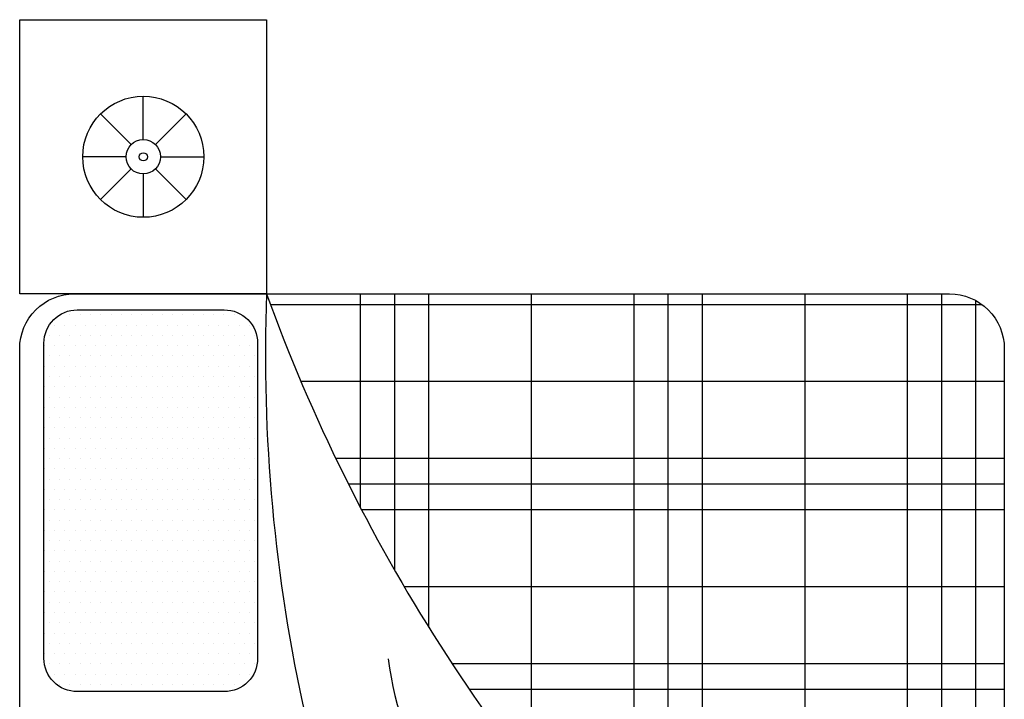
# Model space of a CAD drawing. Units: inches. Extents: x 528 to 2520, y -151 to 1354.
# Tile 33 of 41: x 2171 to 2226, y 770 to 808. Entities that reach past the tile are written whole.
import ezdxf

# ---------------------------------------------------------------- set-up
doc = ezdxf.new("R2010")
doc.units = ezdxf.units.IN
doc.header["$MEASUREMENT"] = 0
doc.layers.add('A-FURN', color=8, linetype='Continuous', lineweight=18)
doc.layers.add('BLOCK', color=6, linetype='Continuous')

# ---------------------------------------------------------------- blocks, each defined once
blk = doc.blocks.new('*X15')
at = {"color": 0}
for p, q in [((276.598, 451.25), (280.51, 451.25)), ((275.455, 450.625), (280.51, 450.625)), ((274.411, 450), (280.51, 450)), ((265.51, 448.125), (267.634, 448.125)), ((271.723, 448.125), (280.51, 448.125)), ((265.51, 446.25), (268.465, 446.25)), ((269.519, 446.25), (280.51, 446.25)), ((265.51, 445.625), (268.531, 445.625)), ((268.866, 445.625), (280.51, 445.625)), ((265.51, 445), (280.51, 445)), ((265.51, 443.125), (280.51, 443.125)), ((265.51, 441.25), (280.51, 441.25)), ((265.51, 440.625), (280.51, 440.625)), ((265.634, 440), (280.386, 440))]:
    blk.add_line(p, q, dxfattribs=at)
blk = doc.blocks.new('*X16')
at = {"color": 0}
for p, q in [((280.312, 439.886), (280.312, 452.896)), ((278.906, 439.482), (278.906, 452.338)), ((277.5, 439.482), (277.5, 451.702)), ((277.031, 439.482), (277.031, 451.471)), ((276.562, 439.482), (276.562, 451.231)), ((275.156, 439.482), (275.156, 450.451)), ((265.781, 439.797), (265.781, 449.511)), ((273.75, 439.482), (273.75, 449.576)), ((266.25, 439.517), (266.25, 449.296)), ((273.281, 439.482), (273.281, 449.261)), ((272.812, 439.482), (272.812, 448.934)), ((267.656, 439.482), (267.656, 448.095)), ((271.406, 439.482), (271.406, 447.876)), ((270, 439.482), (270, 446.689)), ((269.531, 439.482), (269.531, 446.262)), ((269.062, 439.482), (269.062, 445.817))]:
    blk.add_line(p, q, dxfattribs=at)
blk = doc.blocks.new('*X17')
at = {"color": 0}
for p, q in [((273.9375, 457.03125), (273.9375, 457.03125)), ((274.3125, 457.03125), (274.3125, 457.03125)), ((274.6875, 457.03125), (274.6875, 457.03125)), ((275.0625, 457.03125), (275.0625, 457.03125)), ((275.4375, 457.03125), (275.4375, 457.03125)), ((275.8125, 457.03125), (275.8125, 457.03125)), ((276.1875, 457.03125), (276.1875, 457.03125)), ((276.5625, 457.03125), (276.5625, 457.03125)), ((276.9375, 457.03125), (276.9375, 457.03125)), ((277.3125, 457.03125), (277.3125, 457.03125)), ((277.6875, 457.03125), (277.6875, 457.03125)), ((278.0625, 457.03125), (278.0625, 457.03125)), ((278.4375, 457.03125), (278.4375, 457.03125)), ((278.8125, 457.03125), (278.8125, 457.03125)), ((279.1875, 457.03125), (279.1875, 457.03125)), ((279.5625, 457.03125), (279.5625, 457.03125)), ((273.5625, 456.84375), (273.5625, 456.84375)), ((273.75, 456.9375), (273.75, 456.9375)), ((273.9375, 456.84375), (273.9375, 456.84375)), ((274.125, 456.9375), (274.125, 456.9375)), ((274.3125, 456.84375), (274.3125, 456.84375)), ((274.5, 456.9375), (274.5, 456.9375)), ((274.6875, 456.84375), (274.6875, 456.84375)), ((274.875, 456.9375), (274.875, 456.9375)), ((275.0625, 456.84375), (275.0625, 456.84375)), ((275.25, 456.9375), (275.25, 456.9375)), ((275.4375, 456.84375), (275.4375, 456.84375)), ((275.625, 456.9375), (275.625, 456.9375)), ((275.8125, 456.84375), (275.8125, 456.84375)), ((276, 456.9375), (276, 456.9375)), ((276.1875, 456.84375), (276.1875, 456.84375)), ((276.375, 456.9375), (276.375, 456.9375)), ((276.5625, 456.84375), (276.5625, 456.84375)), ((276.75, 456.9375), (276.75, 456.9375)), ((276.9375, 456.84375), (276.9375, 456.84375)), ((277.125, 456.9375), (277.125, 456.9375)), ((277.3125, 456.84375), (277.3125, 456.84375)), ((277.5, 456.9375), (277.5, 456.9375)), ((277.6875, 456.84375), (277.6875, 456.84375)), ((277.875, 456.9375), (277.875, 456.9375)), ((278.0625, 456.84375), (278.0625, 456.84375)), ((278.25, 456.9375), (278.25, 456.9375)), ((278.4375, 456.84375), (278.4375, 456.84375)), ((278.625, 456.9375), (278.625, 456.9375)), ((278.8125, 456.84375), (278.8125, 456.84375)), ((279, 456.9375), (279, 456.9375)), ((279.1875, 456.84375), (279.1875, 456.84375)), ((279.375, 456.9375), (279.375, 456.9375)), ((279.5625, 456.84375), (279.5625, 456.84375)), ((279.75, 456.9375), (279.75, 456.9375)), ((279.9375, 456.84375), (279.9375, 456.84375)), ((273.375, 456.75), (273.375, 456.75)), ((273.75, 456.75), (273.75, 456.75)), ((274.125, 456.75), (274.125, 456.75)), ((274.5, 456.75), (274.5, 456.75)), ((274.875, 456.75), (274.875, 456.75)), ((275.25, 456.75), (275.25, 456.75)), ((275.625, 456.75), (275.625, 456.75)), ((276, 456.75), (276, 456.75)), ((276.375, 456.75), (276.375, 456.75)), ((276.75, 456.75), (276.75, 456.75)), ((277.125, 456.75), (277.125, 456.75)), ((277.5, 456.75), (277.5, 456.75)), ((277.875, 456.75), (277.875, 456.75)), ((278.25, 456.75), (278.25, 456.75)), ((278.625, 456.75), (278.625, 456.75)), ((279, 456.75), (279, 456.75)), ((279.375, 456.75), (279.375, 456.75)), ((279.75, 456.75), (279.75, 456.75)), ((280.125, 456.75), (280.125, 456.75)), ((273.375, 456.5625), (273.375, 456.5625)), ((273.5625, 456.65625), (273.5625, 456.65625)), ((273.75, 456.5625), (273.75, 456.5625)), ((273.9375, 456.65625), (273.9375, 456.65625)), ((274.125, 456.5625), (274.125, 456.5625)), ((274.3125, 456.65625), (274.3125, 456.65625)), ((274.5, 456.5625), (274.5, 456.5625)), ((274.6875, 456.65625), (274.6875, 456.65625)), ((274.875, 456.5625), (274.875, 456.5625)), ((275.0625, 456.65625), (275.0625, 456.65625)), ((275.25, 456.5625), (275.25, 456.5625)), ((275.4375, 456.65625), (275.4375, 456.65625)), ((275.625, 456.5625), (275.625, 456.5625)), ((275.8125, 456.65625), (275.8125, 456.65625)), ((276, 456.5625), (276, 456.5625)), ((276.1875, 456.65625), (276.1875, 456.65625)), ((276.375, 456.5625), (276.375, 456.5625)), ((276.5625, 456.65625), (276.5625, 456.65625)), ((276.75, 456.5625), (276.75, 456.5625)), ((276.9375, 456.65625), (276.9375, 456.65625)), ((277.125, 456.5625), (277.125, 456.5625)), ((277.3125, 456.65625), (277.3125, 456.65625)), ((277.5, 456.5625), (277.5, 456.5625)), ((277.6875, 456.65625), (277.6875, 456.65625)), ((277.875, 456.5625), (277.875, 456.5625)), ((278.0625, 456.65625), (278.0625, 456.65625)), ((278.25, 456.5625), (278.25, 456.5625)), ((278.4375, 456.65625), (278.4375, 456.65625)), ((278.625, 456.5625), (278.625, 456.5625)), ((278.8125, 456.65625), (278.8125, 456.65625)), ((279, 456.5625), (279, 456.5625)), ((279.1875, 456.65625), (279.1875, 456.65625)), ((279.375, 456.5625), (279.375, 456.5625)), ((279.5625, 456.65625), (279.5625, 456.65625)), ((279.75, 456.5625), (279.75, 456.5625)), ((279.9375, 456.65625), (279.9375, 456.65625)), ((280.125, 456.5625), (280.125, 456.5625)), ((273.375, 456.375), (273.375, 456.375)), ((273.5625, 456.46875), (273.5625, 456.46875)), ((273.75, 456.375), (273.75, 456.375)), ((273.9375, 456.46875), (273.9375, 456.46875)), ((274.125, 456.375), (274.125, 456.375)), ((274.3125, 456.46875), (274.3125, 456.46875)), ((274.5, 456.375), (274.5, 456.375)), ((274.6875, 456.46875), (274.6875, 456.46875)), ((274.875, 456.375), (274.875, 456.375)), ((275.0625, 456.46875), (275.0625, 456.46875)), ((275.25, 456.375), (275.25, 456.375)), ((275.4375, 456.46875), (275.4375, 456.46875)), ((275.625, 456.375), (275.625, 456.375)), ((275.8125, 456.46875), (275.8125, 456.46875)), ((276, 456.375), (276, 456.375)), ((276.1875, 456.46875), (276.1875, 456.46875)), ((276.375, 456.375), (276.375, 456.375)), ((276.5625, 456.46875), (276.5625, 456.46875)), ((276.75, 456.375), (276.75, 456.375)), ((276.9375, 456.46875), (276.9375, 456.46875)), ((277.125, 456.375), (277.125, 456.375)), ((277.3125, 456.46875), (277.3125, 456.46875)), ((277.5, 456.375), (277.5, 456.375)), ((277.6875, 456.46875), (277.6875, 456.46875)), ((277.875, 456.375), (277.875, 456.375)), ((278.0625, 456.46875), (278.0625, 456.46875)), ((278.25, 456.375), (278.25, 456.375)), ((278.4375, 456.46875), (278.4375, 456.46875)), ((278.625, 456.375), (278.625, 456.375)), ((278.8125, 456.46875), (278.8125, 456.46875)), ((279, 456.375), (279, 456.375)), ((279.1875, 456.46875), (279.1875, 456.46875)), ((279.375, 456.375), (279.375, 456.375)), ((279.5625, 456.46875), (279.5625, 456.46875)), ((279.75, 456.375), (279.75, 456.375)), ((279.9375, 456.46875), (279.9375, 456.46875)), ((280.125, 456.375), (280.125, 456.375)), ((273.375, 456.1875), (273.375, 456.1875)), ((273.5625, 456.28125), (273.5625, 456.28125)), ((273.75, 456.1875), (273.75, 456.1875)), ((273.9375, 456.28125), (273.9375, 456.28125)), ((274.125, 456.1875), (274.125, 456.1875)), ((274.3125, 456.28125), (274.3125, 456.28125)), ((274.5, 456.1875), (274.5, 456.1875)), ((274.6875, 456.28125), (274.6875, 456.28125)), ((274.875, 456.1875), (274.875, 456.1875)), ((275.0625, 456.28125), (275.0625, 456.28125)), ((275.25, 456.1875), (275.25, 456.1875)), ((275.4375, 456.28125), (275.4375, 456.28125)), ((275.625, 456.1875), (275.625, 456.1875)), ((275.8125, 456.28125), (275.8125, 456.28125)), ((276, 456.1875), (276, 456.1875)), ((276.1875, 456.28125), (276.1875, 456.28125)), ((276.375, 456.1875), (276.375, 456.1875)), ((276.5625, 456.28125), (276.5625, 456.28125)), ((276.75, 456.1875), (276.75, 456.1875)), ((276.9375, 456.28125), (276.9375, 456.28125)), ((277.125, 456.1875), (277.125, 456.1875)), ((277.3125, 456.28125), (277.3125, 456.28125)), ((277.5, 456.1875), (277.5, 456.1875)), ((277.6875, 456.28125), (277.6875, 456.28125)), ((277.875, 456.1875), (277.875, 456.1875)), ((278.0625, 456.28125), (278.0625, 456.28125)), ((278.25, 456.1875), (278.25, 456.1875)), ((278.4375, 456.28125), (278.4375, 456.28125)), ((278.625, 456.1875), (278.625, 456.1875)), ((278.8125, 456.28125), (278.8125, 456.28125)), ((279, 456.1875), (279, 456.1875)), ((279.1875, 456.28125), (279.1875, 456.28125)), ((279.375, 456.1875), (279.375, 456.1875)), ((279.5625, 456.28125), (279.5625, 456.28125)), ((279.75, 456.1875), (279.75, 456.1875)), ((279.9375, 456.28125), (279.9375, 456.28125)), ((280.125, 456.1875), (280.125, 456.1875)), ((273.375, 456), (273.375, 456)), ((273.5625, 456.09375), (273.5625, 456.09375)), ((273.75, 456), (273.75, 456)), ((273.9375, 456.09375), (273.9375, 456.09375)), ((274.125, 456), (274.125, 456)), ((274.3125, 456.09375), (274.3125, 456.09375)), ((274.5, 456), (274.5, 456)), ((274.6875, 456.09375), (274.6875, 456.09375)), ((274.875, 456), (274.875, 456)), ((275.0625, 456.09375), (275.0625, 456.09375)), ((275.25, 456), (275.25, 456)), ((275.4375, 456.09375), (275.4375, 456.09375)), ((275.625, 456), (275.625, 456)), ((275.8125, 456.09375), (275.8125, 456.09375)), ((276, 456), (276, 456)), ((276.1875, 456.09375), (276.1875, 456.09375)), ((276.375, 456), (276.375, 456)), ((276.5625, 456.09375), (276.5625, 456.09375)), ((276.75, 456), (276.75, 456)), ((276.9375, 456.09375), (276.9375, 456.09375)), ((277.125, 456), (277.125, 456)), ((277.3125, 456.09375), (277.3125, 456.09375)), ((277.5, 456), (277.5, 456)), ((277.6875, 456.09375), (277.6875, 456.09375)), ((277.875, 456), (277.875, 456)), ((278.0625, 456.09375), (278.0625, 456.09375)), ((278.25, 456), (278.25, 456)), ((278.4375, 456.09375), (278.4375, 456.09375)), ((278.625, 456), (278.625, 456)), ((278.8125, 456.09375), (278.8125, 456.09375)), ((279, 456), (279, 456)), ((279.1875, 456.09375), (279.1875, 456.09375)), ((279.375, 456), (279.375, 456)), ((279.5625, 456.09375), (279.5625, 456.09375)), ((279.75, 456), (279.75, 456)), ((279.9375, 456.09375), (279.9375, 456.09375)), ((280.125, 456), (280.125, 456)), ((273.375, 455.8125), (273.375, 455.8125)), ((273.5625, 455.90625), (273.5625, 455.90625)), ((273.75, 455.8125), (273.75, 455.8125)), ((273.9375, 455.90625), (273.9375, 455.90625)), ((274.125, 455.8125), (274.125, 455.8125)), ((274.3125, 455.90625), (274.3125, 455.90625)), ((274.5, 455.8125), (274.5, 455.8125)), ((274.6875, 455.90625), (274.6875, 455.90625)), ((274.875, 455.8125), (274.875, 455.8125)), ((275.0625, 455.90625), (275.0625, 455.90625)), ((275.25, 455.8125), (275.25, 455.8125)), ((275.4375, 455.90625), (275.4375, 455.90625)), ((275.625, 455.8125), (275.625, 455.8125)), ((275.8125, 455.90625), (275.8125, 455.90625)), ((276, 455.8125), (276, 455.8125)), ((276.1875, 455.90625), (276.1875, 455.90625)), ((276.375, 455.8125), (276.375, 455.8125)), ((276.5625, 455.90625), (276.5625, 455.90625)), ((276.75, 455.8125), (276.75, 455.8125)), ((276.9375, 455.90625), (276.9375, 455.90625)), ((277.125, 455.8125), (277.125, 455.8125)), ((277.3125, 455.90625), (277.3125, 455.90625)), ((277.5, 455.8125), (277.5, 455.8125)), ((277.6875, 455.90625), (277.6875, 455.90625)), ((277.875, 455.8125), (277.875, 455.8125)), ((278.0625, 455.90625), (278.0625, 455.90625)), ((278.25, 455.8125), (278.25, 455.8125)), ((278.4375, 455.90625), (278.4375, 455.90625)), ((278.625, 455.8125), (278.625, 455.8125)), ((278.8125, 455.90625), (278.8125, 455.90625)), ((279, 455.8125), (279, 455.8125)), ((279.1875, 455.90625), (279.1875, 455.90625)), ((279.375, 455.8125), (279.375, 455.8125)), ((279.5625, 455.90625), (279.5625, 455.90625)), ((279.75, 455.8125), (279.75, 455.8125)), ((279.9375, 455.90625), (279.9375, 455.90625)), ((280.125, 455.8125), (280.125, 455.8125)), ((273.375, 455.625), (273.375, 455.625)), ((273.5625, 455.71875), (273.5625, 455.71875)), ((273.75, 455.625), (273.75, 455.625)), ((273.9375, 455.71875), (273.9375, 455.71875)), ((274.125, 455.625), (274.125, 455.625)), ((274.3125, 455.71875), (274.3125, 455.71875)), ((274.5, 455.625), (274.5, 455.625)), ((274.6875, 455.71875), (274.6875, 455.71875)), ((274.875, 455.625), (274.875, 455.625)), ((275.0625, 455.71875), (275.0625, 455.71875)), ((275.25, 455.625), (275.25, 455.625)), ((275.4375, 455.71875), (275.4375, 455.71875)), ((275.625, 455.625), (275.625, 455.625)), ((275.8125, 455.71875), (275.8125, 455.71875)), ((276, 455.625), (276, 455.625)), ((276.1875, 455.71875), (276.1875, 455.71875)), ((276.375, 455.625), (276.375, 455.625)), ((276.5625, 455.71875), (276.5625, 455.71875)), ((276.75, 455.625), (276.75, 455.625)), ((276.9375, 455.71875), (276.9375, 455.71875)), ((277.125, 455.625), (277.125, 455.625)), ((277.3125, 455.71875), (277.3125, 455.71875)), ((277.5, 455.625), (277.5, 455.625)), ((277.6875, 455.71875), (277.6875, 455.71875)), ((277.875, 455.625), (277.875, 455.625)), ((278.0625, 455.71875), (278.0625, 455.71875)), ((278.25, 455.625), (278.25, 455.625)), ((278.4375, 455.71875), (278.4375, 455.71875)), ((278.625, 455.625), (278.625, 455.625)), ((278.8125, 455.71875), (278.8125, 455.71875)), ((279, 455.625), (279, 455.625)), ((279.1875, 455.71875), (279.1875, 455.71875)), ((279.375, 455.625), (279.375, 455.625)), ((279.5625, 455.71875), (279.5625, 455.71875)), ((279.75, 455.625), (279.75, 455.625)), ((279.9375, 455.71875), (279.9375, 455.71875)), ((280.125, 455.625), (280.125, 455.625)), ((273.375, 455.4375), (273.375, 455.4375)), ((273.5625, 455.53125), (273.5625, 455.53125)), ((273.75, 455.4375), (273.75, 455.4375)), ((273.9375, 455.53125), (273.9375, 455.53125)), ((274.125, 455.4375), (274.125, 455.4375)), ((274.3125, 455.53125), (274.3125, 455.53125)), ((274.5, 455.4375), (274.5, 455.4375)), ((274.6875, 455.53125), (274.6875, 455.53125)), ((274.875, 455.4375), (274.875, 455.4375)), ((275.0625, 455.53125), (275.0625, 455.53125)), ((275.25, 455.4375), (275.25, 455.4375)), ((275.4375, 455.53125), (275.4375, 455.53125)), ((275.625, 455.4375), (275.625, 455.4375)), ((275.8125, 455.53125), (275.8125, 455.53125)), ((276, 455.4375), (276, 455.4375)), ((276.1875, 455.53125), (276.1875, 455.53125)), ((276.375, 455.4375), (276.375, 455.4375)), ((276.5625, 455.53125), (276.5625, 455.53125)), ((276.75, 455.4375), (276.75, 455.4375)), ((276.9375, 455.53125), (276.9375, 455.53125)), ((277.125, 455.4375), (277.125, 455.4375)), ((277.3125, 455.53125), (277.3125, 455.53125)), ((277.5, 455.4375), (277.5, 455.4375)), ((277.6875, 455.53125), (277.6875, 455.53125)), ((277.875, 455.4375), (277.875, 455.4375)), ((278.0625, 455.53125), (278.0625, 455.53125)), ((278.25, 455.4375), (278.25, 455.4375)), ((278.4375, 455.53125), (278.4375, 455.53125)), ((278.625, 455.4375), (278.625, 455.4375)), ((278.8125, 455.53125), (278.8125, 455.53125)), ((279, 455.4375), (279, 455.4375)), ((279.1875, 455.53125), (279.1875, 455.53125)), ((279.375, 455.4375), (279.375, 455.4375)), ((279.5625, 455.53125), (279.5625, 455.53125)), ((279.75, 455.4375), (279.75, 455.4375)), ((279.9375, 455.53125), (279.9375, 455.53125)), ((280.125, 455.4375), (280.125, 455.4375)), ((273.375, 455.25), (273.375, 455.25)), ((273.5625, 455.34375), (273.5625, 455.34375)), ((273.75, 455.25), (273.75, 455.25)), ((273.9375, 455.34375), (273.9375, 455.34375)), ((274.125, 455.25), (274.125, 455.25)), ((274.3125, 455.34375), (274.3125, 455.34375)), ((274.5, 455.25), (274.5, 455.25)), ((274.6875, 455.34375), (274.6875, 455.34375)), ((274.875, 455.25), (274.875, 455.25)), ((275.0625, 455.34375), (275.0625, 455.34375)), ((275.25, 455.25), (275.25, 455.25)), ((275.4375, 455.34375), (275.4375, 455.34375)), ((275.625, 455.25), (275.625, 455.25)), ((275.8125, 455.34375), (275.8125, 455.34375)), ((276, 455.25), (276, 455.25)), ((276.1875, 455.34375), (276.1875, 455.34375)), ((276.375, 455.25), (276.375, 455.25)), ((276.5625, 455.34375), (276.5625, 455.34375)), ((276.75, 455.25), (276.75, 455.25)), ((276.9375, 455.34375), (276.9375, 455.34375)), ((277.125, 455.25), (277.125, 455.25)), ((277.3125, 455.34375), (277.3125, 455.34375)), ((277.5, 455.25), (277.5, 455.25)), ((277.6875, 455.34375), (277.6875, 455.34375)), ((277.875, 455.25), (277.875, 455.25)), ((278.0625, 455.34375), (278.0625, 455.34375)), ((278.25, 455.25), (278.25, 455.25)), ((278.4375, 455.34375), (278.4375, 455.34375)), ((278.625, 455.25), (278.625, 455.25)), ((278.8125, 455.34375), (278.8125, 455.34375)), ((279, 455.25), (279, 455.25)), ((279.1875, 455.34375), (279.1875, 455.34375)), ((279.375, 455.25), (279.375, 455.25)), ((279.5625, 455.34375), (279.5625, 455.34375)), ((279.75, 455.25), (279.75, 455.25)), ((279.9375, 455.34375), (279.9375, 455.34375)), ((280.125, 455.25), (280.125, 455.25)), ((273.375, 455.0625), (273.375, 455.0625)), ((273.5625, 455.15625), (273.5625, 455.15625)), ((273.75, 455.0625), (273.75, 455.0625)), ((273.9375, 455.15625), (273.9375, 455.15625)), ((274.125, 455.0625), (274.125, 455.0625)), ((274.3125, 455.15625), (274.3125, 455.15625)), ((274.5, 455.0625), (274.5, 455.0625)), ((274.6875, 455.15625), (274.6875, 455.15625)), ((274.875, 455.0625), (274.875, 455.0625)), ((275.0625, 455.15625), (275.0625, 455.15625)), ((275.25, 455.0625), (275.25, 455.0625)), ((275.4375, 455.15625), (275.4375, 455.15625)), ((275.625, 455.0625), (275.625, 455.0625)), ((275.8125, 455.15625), (275.8125, 455.15625)), ((276, 455.0625), (276, 455.0625)), ((276.1875, 455.15625), (276.1875, 455.15625)), ((276.375, 455.0625), (276.375, 455.0625)), ((276.5625, 455.15625), (276.5625, 455.15625)), ((276.75, 455.0625), (276.75, 455.0625)), ((276.9375, 455.15625), (276.9375, 455.15625)), ((277.125, 455.0625), (277.125, 455.0625)), ((277.3125, 455.15625), (277.3125, 455.15625)), ((277.5, 455.0625), (277.5, 455.0625)), ((277.6875, 455.15625), (277.6875, 455.15625)), ((277.875, 455.0625), (277.875, 455.0625)), ((278.0625, 455.15625), (278.0625, 455.15625)), ((278.25, 455.0625), (278.25, 455.0625)), ((278.4375, 455.15625), (278.4375, 455.15625)), ((278.625, 455.0625), (278.625, 455.0625)), ((278.8125, 455.15625), (278.8125, 455.15625)), ((279, 455.0625), (279, 455.0625)), ((279.1875, 455.15625), (279.1875, 455.15625)), ((279.375, 455.0625), (279.375, 455.0625)), ((279.5625, 455.15625), (279.5625, 455.15625)), ((279.75, 455.0625), (279.75, 455.0625)), ((279.9375, 455.15625), (279.9375, 455.15625)), ((280.125, 455.0625), (280.125, 455.0625)), ((273.375, 454.875), (273.375, 454.875)), ((273.5625, 454.96875), (273.5625, 454.96875)), ((273.75, 454.875), (273.75, 454.875)), ((273.9375, 454.96875), (273.9375, 454.96875)), ((274.125, 454.875), (274.125, 454.875)), ((274.3125, 454.96875), (274.3125, 454.96875)), ((274.5, 454.875), (274.5, 454.875)), ((274.6875, 454.96875), (274.6875, 454.96875)), ((274.875, 454.875), (274.875, 454.875)), ((275.0625, 454.96875), (275.0625, 454.96875)), ((275.25, 454.875), (275.25, 454.875)), ((275.4375, 454.96875), (275.4375, 454.96875)), ((275.625, 454.875), (275.625, 454.875)), ((275.8125, 454.96875), (275.8125, 454.96875)), ((276, 454.875), (276, 454.875)), ((276.1875, 454.96875), (276.1875, 454.96875)), ((276.375, 454.875), (276.375, 454.875)), ((276.5625, 454.96875), (276.5625, 454.96875)), ((276.75, 454.875), (276.75, 454.875)), ((276.9375, 454.96875), (276.9375, 454.96875)), ((277.125, 454.875), (277.125, 454.875)), ((277.3125, 454.96875), (277.3125, 454.96875)), ((277.5, 454.875), (277.5, 454.875)), ((277.6875, 454.96875), (277.6875, 454.96875)), ((277.875, 454.875), (277.875, 454.875)), ((278.0625, 454.96875), (278.0625, 454.96875)), ((278.25, 454.875), (278.25, 454.875)), ((278.4375, 454.96875), (278.4375, 454.96875)), ((278.625, 454.875), (278.625, 454.875)), ((278.8125, 454.96875), (278.8125, 454.96875)), ((279, 454.875), (279, 454.875)), ((279.1875, 454.96875), (279.1875, 454.96875)), ((279.375, 454.875), (279.375, 454.875)), ((279.5625, 454.96875), (279.5625, 454.96875)), ((279.75, 454.875), (279.75, 454.875)), ((279.9375, 454.96875), (279.9375, 454.96875)), ((280.125, 454.875), (280.125, 454.875)), ((273.375, 454.6875), (273.375, 454.6875)), ((273.5625, 454.78125), (273.5625, 454.78125)), ((273.75, 454.6875), (273.75, 454.6875)), ((273.9375, 454.78125), (273.9375, 454.78125)), ((274.125, 454.6875), (274.125, 454.6875)), ((274.3125, 454.78125), (274.3125, 454.78125)), ((274.5, 454.6875), (274.5, 454.6875)), ((274.6875, 454.78125), (274.6875, 454.78125)), ((274.875, 454.6875), (274.875, 454.6875)), ((275.0625, 454.78125), (275.0625, 454.78125)), ((275.25, 454.6875), (275.25, 454.6875)), ((275.4375, 454.78125), (275.4375, 454.78125)), ((275.625, 454.6875), (275.625, 454.6875)), ((275.8125, 454.78125), (275.8125, 454.78125)), ((276, 454.6875), (276, 454.6875)), ((276.1875, 454.78125), (276.1875, 454.78125)), ((276.375, 454.6875), (276.375, 454.6875)), ((276.5625, 454.78125), (276.5625, 454.78125)), ((276.75, 454.6875), (276.75, 454.6875)), ((276.9375, 454.78125), (276.9375, 454.78125)), ((277.125, 454.6875), (277.125, 454.6875)), ((277.3125, 454.78125), (277.3125, 454.78125)), ((277.5, 454.6875), (277.5, 454.6875)), ((277.6875, 454.78125), (277.6875, 454.78125)), ((277.875, 454.6875), (277.875, 454.6875)), ((278.0625, 454.78125), (278.0625, 454.78125)), ((278.25, 454.6875), (278.25, 454.6875)), ((278.4375, 454.78125), (278.4375, 454.78125)), ((278.625, 454.6875), (278.625, 454.6875)), ((278.8125, 454.78125), (278.8125, 454.78125)), ((279, 454.6875), (279, 454.6875)), ((279.1875, 454.78125), (279.1875, 454.78125)), ((279.375, 454.6875), (279.375, 454.6875)), ((279.5625, 454.78125), (279.5625, 454.78125)), ((279.75, 454.6875), (279.75, 454.6875)), ((279.9375, 454.78125), (279.9375, 454.78125)), ((280.125, 454.6875), (280.125, 454.6875)), ((273.5625, 454.59375), (273.5625, 454.59375)), ((273.9375, 454.59375), (273.9375, 454.59375)), ((274.3125, 454.59375), (274.3125, 454.59375)), ((274.6875, 454.59375), (274.6875, 454.59375)), ((275.0625, 454.59375), (275.0625, 454.59375)), ((275.4375, 454.59375), (275.4375, 454.59375)), ((275.8125, 454.59375), (275.8125, 454.59375)), ((276.1875, 454.59375), (276.1875, 454.59375)), ((276.5625, 454.59375), (276.5625, 454.59375)), ((276.9375, 454.59375), (276.9375, 454.59375)), ((277.3125, 454.59375), (277.3125, 454.59375)), ((277.6875, 454.59375), (277.6875, 454.59375)), ((278.0625, 454.59375), (278.0625, 454.59375)), ((278.4375, 454.59375), (278.4375, 454.59375)), ((278.8125, 454.59375), (278.8125, 454.59375)), ((279.1875, 454.59375), (279.1875, 454.59375)), ((279.5625, 454.59375), (279.5625, 454.59375)), ((279.9375, 454.59375), (279.9375, 454.59375)), ((273.375, 454.5), (273.375, 454.5)), ((273.5625, 454.40625), (273.5625, 454.40625)), ((273.75, 454.5), (273.75, 454.5)), ((273.9375, 454.40625), (273.9375, 454.40625)), ((274.125, 454.5), (274.125, 454.5)), ((274.3125, 454.40625), (274.3125, 454.40625)), ((274.5, 454.5), (274.5, 454.5)), ((274.6875, 454.40625), (274.6875, 454.40625)), ((274.875, 454.5), (274.875, 454.5)), ((275.0625, 454.40625), (275.0625, 454.40625)), ((275.25, 454.5), (275.25, 454.5)), ((275.4375, 454.40625), (275.4375, 454.40625)), ((275.625, 454.5), (275.625, 454.5)), ((275.8125, 454.40625), (275.8125, 454.40625)), ((276, 454.5), (276, 454.5)), ((276.1875, 454.40625), (276.1875, 454.40625)), ((276.375, 454.5), (276.375, 454.5)), ((276.5625, 454.40625), (276.5625, 454.40625)), ((276.75, 454.5), (276.75, 454.5)), ((276.9375, 454.40625), (276.9375, 454.40625)), ((277.125, 454.5), (277.125, 454.5)), ((277.3125, 454.40625), (277.3125, 454.40625)), ((277.5, 454.5), (277.5, 454.5)), ((277.6875, 454.40625), (277.6875, 454.40625)), ((277.875, 454.5), (277.875, 454.5)), ((278.0625, 454.40625), (278.0625, 454.40625)), ((278.25, 454.5), (278.25, 454.5)), ((278.4375, 454.40625), (278.4375, 454.40625)), ((278.625, 454.5), (278.625, 454.5)), ((278.8125, 454.40625), (278.8125, 454.40625)), ((279, 454.5), (279, 454.5)), ((279.1875, 454.40625), (279.1875, 454.40625)), ((279.375, 454.5), (279.375, 454.5)), ((279.5625, 454.40625), (279.5625, 454.40625)), ((279.75, 454.5), (279.75, 454.5)), ((279.9375, 454.40625), (279.9375, 454.40625)), ((280.125, 454.5), (280.125, 454.5)), ((273.375, 454.3125), (273.375, 454.3125)), ((273.5625, 454.21875), (273.5625, 454.21875)), ((273.75, 454.3125), (273.75, 454.3125)), ((273.9375, 454.21875), (273.9375, 454.21875)), ((274.125, 454.3125), (274.125, 454.3125)), ((274.3125, 454.21875), (274.3125, 454.21875)), ((274.5, 454.3125), (274.5, 454.3125)), ((274.6875, 454.21875), (274.6875, 454.21875)), ((274.875, 454.3125), (274.875, 454.3125)), ((275.0625, 454.21875), (275.0625, 454.21875)), ((275.25, 454.3125), (275.25, 454.3125)), ((275.4375, 454.21875), (275.4375, 454.21875)), ((275.625, 454.3125), (275.625, 454.3125)), ((275.8125, 454.21875), (275.8125, 454.21875)), ((276, 454.3125), (276, 454.3125)), ((276.1875, 454.21875), (276.1875, 454.21875)), ((276.375, 454.3125), (276.375, 454.3125)), ((276.5625, 454.21875), (276.5625, 454.21875)), ((276.75, 454.3125), (276.75, 454.3125)), ((276.9375, 454.21875), (276.9375, 454.21875)), ((277.125, 454.3125), (277.125, 454.3125)), ((277.3125, 454.21875), (277.3125, 454.21875)), ((277.5, 454.3125), (277.5, 454.3125)), ((277.6875, 454.21875), (277.6875, 454.21875)), ((277.875, 454.3125), (277.875, 454.3125)), ((278.0625, 454.21875), (278.0625, 454.21875)), ((278.25, 454.3125), (278.25, 454.3125)), ((278.4375, 454.21875), (278.4375, 454.21875)), ((278.625, 454.3125), (278.625, 454.3125)), ((278.8125, 454.21875), (278.8125, 454.21875)), ((279, 454.3125), (279, 454.3125)), ((279.1875, 454.21875), (279.1875, 454.21875)), ((279.375, 454.3125), (279.375, 454.3125)), ((279.5625, 454.21875), (279.5625, 454.21875)), ((279.75, 454.3125), (279.75, 454.3125)), ((279.9375, 454.21875), (279.9375, 454.21875)), ((280.125, 454.3125), (280.125, 454.3125)), ((273.375, 454.125), (273.375, 454.125)), ((273.5625, 454.03125), (273.5625, 454.03125)), ((273.75, 454.125), (273.75, 454.125)), ((273.9375, 454.03125), (273.9375, 454.03125)), ((274.125, 454.125), (274.125, 454.125)), ((274.3125, 454.03125), (274.3125, 454.03125)), ((274.5, 454.125), (274.5, 454.125)), ((274.6875, 454.03125), (274.6875, 454.03125)), ((274.875, 454.125), (274.875, 454.125)), ((275.0625, 454.03125), (275.0625, 454.03125)), ((275.25, 454.125), (275.25, 454.125)), ((275.4375, 454.03125), (275.4375, 454.03125)), ((275.625, 454.125), (275.625, 454.125)), ((275.8125, 454.03125), (275.8125, 454.03125)), ((276, 454.125), (276, 454.125)), ((276.1875, 454.03125), (276.1875, 454.03125)), ((276.375, 454.125), (276.375, 454.125)), ((276.5625, 454.03125), (276.5625, 454.03125)), ((276.75, 454.125), (276.75, 454.125)), ((276.9375, 454.03125), (276.9375, 454.03125)), ((277.125, 454.125), (277.125, 454.125)), ((277.3125, 454.03125), (277.3125, 454.03125)), ((277.5, 454.125), (277.5, 454.125)), ((277.6875, 454.03125), (277.6875, 454.03125)), ((277.875, 454.125), (277.875, 454.125)), ((278.0625, 454.03125), (278.0625, 454.03125)), ((278.25, 454.125), (278.25, 454.125)), ((278.4375, 454.03125), (278.4375, 454.03125)), ((278.625, 454.125), (278.625, 454.125)), ((278.8125, 454.03125), (278.8125, 454.03125)), ((279, 454.125), (279, 454.125)), ((279.1875, 454.03125), (279.1875, 454.03125)), ((279.375, 454.125), (279.375, 454.125)), ((279.5625, 454.03125), (279.5625, 454.03125)), ((279.75, 454.125), (279.75, 454.125)), ((279.9375, 454.03125), (279.9375, 454.03125)), ((280.125, 454.125), (280.125, 454.125)), ((273.375, 453.9375), (273.375, 453.9375)), ((273.5625, 453.84375), (273.5625, 453.84375)), ((273.75, 453.9375), (273.75, 453.9375)), ((273.9375, 453.84375), (273.9375, 453.84375)), ((274.125, 453.9375), (274.125, 453.9375)), ((274.3125, 453.84375), (274.3125, 453.84375)), ((274.5, 453.9375), (274.5, 453.9375)), ((274.6875, 453.84375), (274.6875, 453.84375)), ((274.875, 453.9375), (274.875, 453.9375)), ((275.0625, 453.84375), (275.0625, 453.84375)), ((275.25, 453.9375), (275.25, 453.9375)), ((275.4375, 453.84375), (275.4375, 453.84375)), ((275.625, 453.9375), (275.625, 453.9375)), ((275.8125, 453.84375), (275.8125, 453.84375)), ((276, 453.9375), (276, 453.9375)), ((276.1875, 453.84375), (276.1875, 453.84375)), ((276.375, 453.9375), (276.375, 453.9375)), ((276.5625, 453.84375), (276.5625, 453.84375)), ((276.75, 453.9375), (276.75, 453.9375)), ((276.9375, 453.84375), (276.9375, 453.84375)), ((277.125, 453.9375), (277.125, 453.9375)), ((277.3125, 453.84375), (277.3125, 453.84375)), ((277.5, 453.9375), (277.5, 453.9375)), ((277.6875, 453.84375), (277.6875, 453.84375)), ((277.875, 453.9375), (277.875, 453.9375)), ((278.0625, 453.84375), (278.0625, 453.84375)), ((278.25, 453.9375), (278.25, 453.9375)), ((278.4375, 453.84375), (278.4375, 453.84375)), ((278.625, 453.9375), (278.625, 453.9375)), ((278.8125, 453.84375), (278.8125, 453.84375)), ((279, 453.9375), (279, 453.9375)), ((279.1875, 453.84375), (279.1875, 453.84375)), ((279.375, 453.9375), (279.375, 453.9375)), ((279.5625, 453.84375), (279.5625, 453.84375)), ((279.75, 453.9375), (279.75, 453.9375)), ((279.9375, 453.84375), (279.9375, 453.84375)), ((280.125, 453.9375), (280.125, 453.9375)), ((273.375, 453.75), (273.375, 453.75)), ((273.5625, 453.65625), (273.5625, 453.65625)), ((273.75, 453.75), (273.75, 453.75)), ((273.9375, 453.65625), (273.9375, 453.65625)), ((274.125, 453.75), (274.125, 453.75)), ((274.3125, 453.65625), (274.3125, 453.65625)), ((274.5, 453.75), (274.5, 453.75)), ((274.6875, 453.65625), (274.6875, 453.65625)), ((274.875, 453.75), (274.875, 453.75)), ((275.0625, 453.65625), (275.0625, 453.65625)), ((275.25, 453.75), (275.25, 453.75)), ((275.4375, 453.65625), (275.4375, 453.65625)), ((275.625, 453.75), (275.625, 453.75)), ((275.8125, 453.65625), (275.8125, 453.65625)), ((276, 453.75), (276, 453.75)), ((276.1875, 453.65625), (276.1875, 453.65625)), ((276.375, 453.75), (276.375, 453.75)), ((276.5625, 453.65625), (276.5625, 453.65625)), ((276.75, 453.75), (276.75, 453.75)), ((276.9375, 453.65625), (276.9375, 453.65625)), ((277.125, 453.75), (277.125, 453.75)), ((277.3125, 453.65625), (277.3125, 453.65625)), ((277.5, 453.75), (277.5, 453.75)), ((277.6875, 453.65625), (277.6875, 453.65625)), ((277.875, 453.75), (277.875, 453.75)), ((278.0625, 453.65625), (278.0625, 453.65625)), ((278.25, 453.75), (278.25, 453.75)), ((278.4375, 453.65625), (278.4375, 453.65625)), ((278.625, 453.75), (278.625, 453.75)), ((278.8125, 453.65625), (278.8125, 453.65625)), ((279, 453.75), (279, 453.75)), ((279.1875, 453.65625), (279.1875, 453.65625)), ((279.375, 453.75), (279.375, 453.75)), ((279.5625, 453.65625), (279.5625, 453.65625)), ((279.75, 453.75), (279.75, 453.75)), ((279.9375, 453.65625), (279.9375, 453.65625)), ((280.125, 453.75), (280.125, 453.75)), ((273.375, 453.5625), (273.375, 453.5625)), ((273.5625, 453.46875), (273.5625, 453.46875)), ((273.75, 453.5625), (273.75, 453.5625)), ((273.9375, 453.46875), (273.9375, 453.46875)), ((274.125, 453.5625), (274.125, 453.5625)), ((274.3125, 453.46875), (274.3125, 453.46875)), ((274.5, 453.5625), (274.5, 453.5625)), ((274.6875, 453.46875), (274.6875, 453.46875)), ((274.875, 453.5625), (274.875, 453.5625)), ((275.0625, 453.46875), (275.0625, 453.46875)), ((275.25, 453.5625), (275.25, 453.5625)), ((275.4375, 453.46875), (275.4375, 453.46875)), ((275.625, 453.5625), (275.625, 453.5625)), ((275.8125, 453.46875), (275.8125, 453.46875)), ((276, 453.5625), (276, 453.5625)), ((276.1875, 453.46875), (276.1875, 453.46875)), ((276.375, 453.5625), (276.375, 453.5625)), ((276.5625, 453.46875), (276.5625, 453.46875)), ((276.75, 453.5625), (276.75, 453.5625)), ((276.9375, 453.46875), (276.9375, 453.46875)), ((277.125, 453.5625), (277.125, 453.5625)), ((277.3125, 453.46875), (277.3125, 453.46875)), ((277.5, 453.5625), (277.5, 453.5625)), ((277.6875, 453.46875), (277.6875, 453.46875)), ((277.875, 453.5625), (277.875, 453.5625)), ((278.0625, 453.46875), (278.0625, 453.46875)), ((278.25, 453.5625), (278.25, 453.5625)), ((278.4375, 453.46875), (278.4375, 453.46875)), ((278.625, 453.5625), (278.625, 453.5625)), ((278.8125, 453.46875), (278.8125, 453.46875)), ((279, 453.5625), (279, 453.5625)), ((279.1875, 453.46875), (279.1875, 453.46875)), ((279.375, 453.5625), (279.375, 453.5625)), ((279.5625, 453.46875), (279.5625, 453.46875)), ((279.75, 453.5625), (279.75, 453.5625)), ((279.9375, 453.46875), (279.9375, 453.46875)), ((280.125, 453.5625), (280.125, 453.5625)), ((273.375, 453.375), (273.375, 453.375)), ((273.5625, 453.28125), (273.5625, 453.28125)), ((273.75, 453.375), (273.75, 453.375)), ((273.9375, 453.28125), (273.9375, 453.28125)), ((274.125, 453.375), (274.125, 453.375)), ((274.3125, 453.28125), (274.3125, 453.28125)), ((274.5, 453.375), (274.5, 453.375)), ((274.6875, 453.28125), (274.6875, 453.28125)), ((274.875, 453.375), (274.875, 453.375)), ((275.0625, 453.28125), (275.0625, 453.28125)), ((275.25, 453.375), (275.25, 453.375)), ((275.4375, 453.28125), (275.4375, 453.28125)), ((275.625, 453.375), (275.625, 453.375)), ((275.8125, 453.28125), (275.8125, 453.28125)), ((276, 453.375), (276, 453.375)), ((276.1875, 453.28125), (276.1875, 453.28125)), ((276.375, 453.375), (276.375, 453.375)), ((276.5625, 453.28125), (276.5625, 453.28125)), ((276.75, 453.375), (276.75, 453.375)), ((276.9375, 453.28125), (276.9375, 453.28125)), ((277.125, 453.375), (277.125, 453.375)), ((277.3125, 453.28125), (277.3125, 453.28125)), ((277.5, 453.375), (277.5, 453.375)), ((277.6875, 453.28125), (277.6875, 453.28125)), ((277.875, 453.375), (277.875, 453.375)), ((278.0625, 453.28125), (278.0625, 453.28125)), ((278.25, 453.375), (278.25, 453.375)), ((278.4375, 453.28125), (278.4375, 453.28125)), ((278.625, 453.375), (278.625, 453.375)), ((278.8125, 453.28125), (278.8125, 453.28125)), ((279, 453.375), (279, 453.375)), ((279.1875, 453.28125), (279.1875, 453.28125)), ((279.375, 453.375), (279.375, 453.375)), ((279.5625, 453.28125), (279.5625, 453.28125)), ((279.75, 453.375), (279.75, 453.375)), ((279.9375, 453.28125), (279.9375, 453.28125)), ((273.75, 453.1875), (273.75, 453.1875)), ((274.125, 453.1875), (274.125, 453.1875)), ((274.5, 453.1875), (274.5, 453.1875)), ((274.875, 453.1875), (274.875, 453.1875)), ((275.25, 453.1875), (275.25, 453.1875)), ((275.625, 453.1875), (275.625, 453.1875)), ((276, 453.1875), (276, 453.1875)), ((276.375, 453.1875), (276.375, 453.1875)), ((276.75, 453.1875), (276.75, 453.1875)), ((277.125, 453.1875), (277.125, 453.1875)), ((277.5, 453.1875), (277.5, 453.1875)), ((277.875, 453.1875), (277.875, 453.1875)), ((278.25, 453.1875), (278.25, 453.1875)), ((278.625, 453.1875), (278.625, 453.1875)), ((279, 453.1875), (279, 453.1875)), ((279.375, 453.1875), (279.375, 453.1875)), ((279.75, 453.1875), (279.75, 453.1875))]:
    blk.add_line(p, q, dxfattribs=at)
blk = doc.blocks.new('A$C52E67D0D')
at = {"layer": 'BLOCK'}
for p, q in [((2251.5, 1605.5), (2251.5, 1684.7)), ((2229.3, 1596.3), (2173.3, 1652.3)), ((2273.7, 1596.3), (2329.7, 1652.3)), ((2220.1, 1574.1), (2140.9, 1574.1)), ((2282.9, 1574.1), (2362.1, 1574.1)), ((2229.3, 1551.9), (2173.3, 1495.9)), ((2273.7, 1551.9), (2329.7, 1495.9)), ((2251.5, 1542.8), (2251.5, 1463.5))]:
    blk.add_line(p, q, dxfattribs=at)
for points in [[(1901, 0), (601, 0, -0.414214), (501, 100), (501, 1700, -0.414214), (601, 1800), (1901, 1800, -0.414214), (2001, 1700), (2001, 100, -0.414214)], [(1911, 1365.1), (1335, 1365.1, -0.414214), (1274.2, 1425.9), (1274.2, 1694.8, -0.414214), (1335, 1755.7), (1911, 1755.7, -0.414214), (1971.8, 1694.8), (1971.8, 1425.9, -0.414214)]]:
    blk.add_lwpolyline(points, format="xyb", close=True, dxfattribs=at)
blk.add_lwpolyline([(2001, 1348.6), (2001, 1799.6), (2502, 1799.6), (2502, 1348.6)], close=True, dxfattribs=at)
for radius in [110.6, 31.4, 7.46]:
    blk.add_circle((2251.5, 1574.1), radius, dxfattribs=at)
for centre, radius, start, end in [((1888.6, -1664.5), 3015.3, 87.8642, 117.4001), ((3101, -1685.8), 3227.7, 109.926, 135.3977), ((1410.8, 520.2), 610.8, 97.2157, 147.6656)]:
    blk.add_arc(centre, radius, start, end, dxfattribs=at)
at = {"layer": 'BLOCK', "xscale": 100, "yscale": 100, "zscale": 100}
for name in ['*X17', '*X16', '*X15']:
    blk.add_blockref(name, (-26050, -43948.2), dxfattribs=at)

msp = doc.modelspace()

# ---------------------------------------------------------------- block references
at = {"layer": 'A-FURN', "xscale": 0.0306954436450662, "yscale": 0.0306954436450662, "zscale": 0.0306954436450662, "rotation": 90}
msp.add_blockref('A$C52E67D0D', (2226.437, 731.467), dxfattribs=at)

doc.saveas('drawing.dxf')
